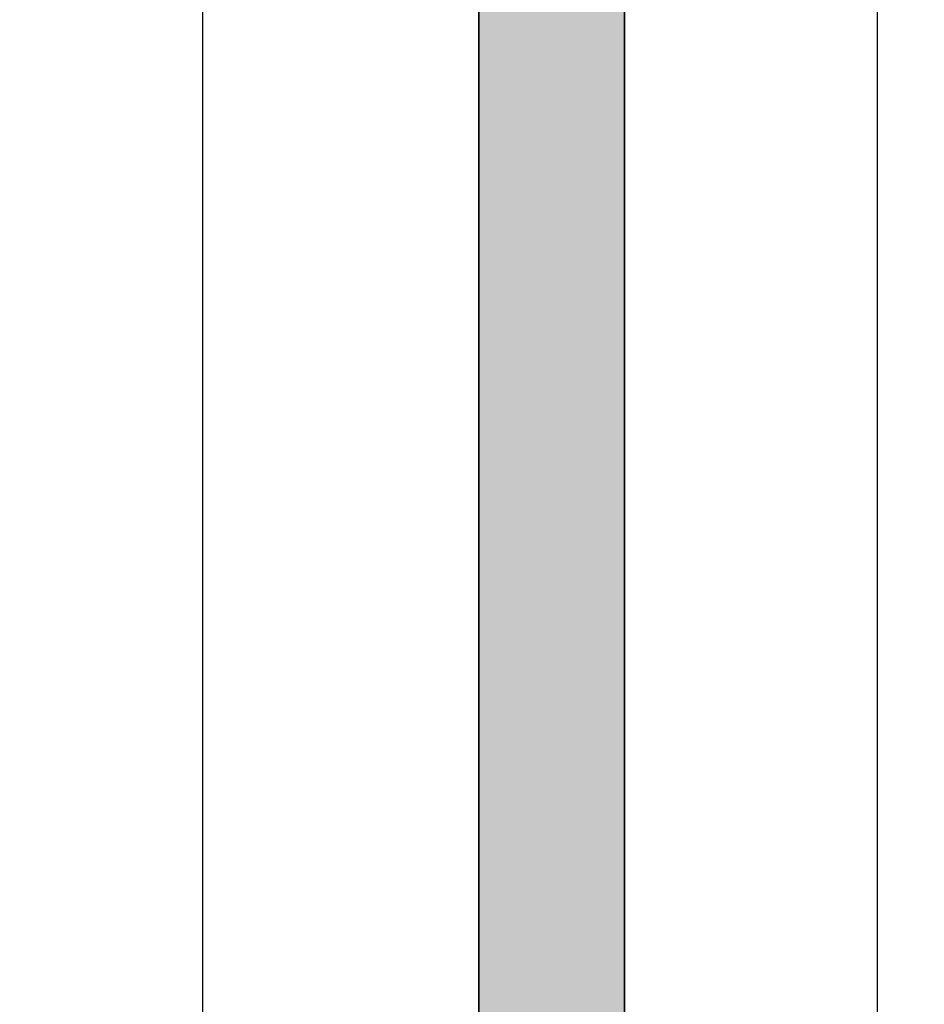
# Model space of a CAD drawing. Units: inches. Extents: x -5 to 330, y -522 to 40.
# Tile 8 of 23: x -5 to 51, y -391 to -330. Entities that reach past the tile are written whole.
import ezdxf

# ---------------------------------------------------------------- set-up
doc = ezdxf.new("R2010")
doc.units = ezdxf.units.IN
doc.header["$MEASUREMENT"] = 0
for name, color, linetype, lineweight in [('A-ANNO-DIMS', 2, 'Continuous', 18), ('A-FLOR-CASE', 8, 'Continuous', 25), ('A-WALL', 7, 'Continuous', 35)]:
    doc.layers.add(name, color=color, linetype=linetype, lineweight=lineweight)
doc.layers.add('A-WALL-PATT', color=18, linetype='Continuous', lineweight=13, true_color=0x000000)
doc.styles.get("Standard").update_dxf_attribs({"font": 'arial.ttf'})
doc.dimstyles.get("Standard").update_dxf_attribs({"dimtxt": 0.18, "dimasz": 0.18, "dimexe": 0.18, "dimexo": 0.0625, "dimgap": 0.09, "dimtad": 0, "dimtih": 1, "dimtoh": 1, "dimdec": 0, "dimzin": 0, "dimdsep": 46, "dimlunit": 3, "dimtxsty": 'Standard', "dimcen": 0.09, "dimadec": 0, "dimazin": 0, "dimtfac": 1, "dimtdec": 0, "dimtofl": 0, "dimtmove": 0, "dimatfit": 3, "dimfxl": 1, "dimtolj": 1, "dimtzin": 0, "dimarcsym": 0})

# ---------------------------------------------------------------- blocks, each defined once
blk = doc.blocks.new('*D2')
at = {"layer": 'A-ANNO-DIMS', "color": 0, "lineweight": -2, "transparency": 16777216}
for p, q in [((23.447, 12.356), (6.274, 12.356)), ((6.454, 12.176), (6.454, -203.738)), ((6.454, -425.964), (6.454, -210.049)), ((23.447, -426.144), (6.274, -426.144))]:
    blk.add_line(p, q, dxfattribs=at)
at = {"layer": 'A-ANNO-DIMS', "color": 0, "transparency": 16777216}
for points in [[(6.424, 12.176), (6.484, 12.176), (6.454, 12.356)], [(6.424, -425.964), (6.484, -425.964), (6.454, -426.144)]]:
    blk.add_solid(points, dxfattribs=at)
at = {"layer": 'Defpoints', "color": 0, "transparency": 16777216}
for p in [(23.51, 12.356), (6.454, -426.144), (23.51, -426.144)]:
    blk.add_point(p, dxfattribs=at)
at = {"layer": 'A-ANNO-DIMS', "color": 0, "transparency": 16777216, "insert": (6.454, -206.894), "char_height": 6, "attachment_point": 5}
blk.add_mtext('\\A1;36\'-7"', dxfattribs=at)
blk = doc.blocks.new('*D40')
at = {"layer": 'A-ANNO-DIMS', "color": 0, "lineweight": -2, "transparency": 16777216}
for p, q in [((32.51, -246.706), (32.51, -522.309)), ((79.01, -246.706), (79.01, -522.309)), ((32.69, -522.129), (55.151, -522.129)), ((78.83, -522.129), (56.369, -522.129))]:
    blk.add_line(p, q, dxfattribs=at)
at = {"layer": 'A-ANNO-DIMS', "color": 0, "transparency": 16777216}
for points in [[(32.69, -522.099), (32.69, -522.159), (32.51, -522.129)], [(78.83, -522.099), (78.83, -522.159), (79.01, -522.129)]]:
    blk.add_solid(points, dxfattribs=at)
at = {"layer": 'Defpoints', "color": 0, "transparency": 16777216}
for p in [(32.51, -246.644), (79.01, -246.644), (79.01, -522.129)]:
    blk.add_point(p, dxfattribs=at)
at = {"layer": 'A-ANNO-DIMS', "color": 0, "transparency": 16777216, "insert": (55.76, -522.129), "char_height": 0.18, "attachment_point": 5}
blk.add_mtext('\\A1;3\'-10 1/2"', dxfattribs=at)

msp = doc.modelspace()

# ---------------------------------------------------------------- hatches: boundary and pattern name
at = {"layer": 'A-WALL-PATT'}
h = msp.add_hatch(color=256, dxfattribs=at)
h.dxf.hatch_style = 1
h.paths.add_polyline_path([(164.01, -44.152), (159.51, -44.152), (159.51, -153.144), (164.01, -153.144)], flags=17)
h.paths.add_polyline_path([(224.01, -188.144), (272.01, -188.144), (272.01, -218.144), (260.01, -218.144), (260.01, -222.644), (272.01, -222.644), (272.01, -292.644), (159.01, -292.644), (159.01, -297.144), (272.01, -297.144), (272.01, -417.144), (245.51, -417.144), (245.51, -426.144), (272.01, -426.144), (272.01, -495.144), (281.01, -495.144), (281.01, 12.356), (23.51, 12.356), (23.51, -426.144), (62.918, -426.144), (62.918, -417.144), (32.51, -417.144), (32.51, -297.144), (48.129, -297.144), (48.129, -292.644), (32.51, -292.644), (32.51, -140.644), (133.51, -140.644), (133.51, -131.644), (32.51, -131.644), (32.51, 3.356), (159.51, 3.356), (164.01, 3.356), (220.01, 3.356), (224.51, 3.356), (272.01, 3.356), (272.01, -179.144), (159.51, -179.144), (159.51, -188.144), (219.51, -188.144), (219.51, -266.644), (224.01, -266.644), (224.01, -222.644), (236.01, -222.644), (236.01, -218.144), (224.01, -218.144)])
h.paths.add_polyline_path([(133.01, -292.644), (128.51, -292.644), (128.51, -297.144), (128.51, -417.144), (122.918, -417.144), (122.918, -426.144), (133.01, -426.144)], flags=17)
h.paths.add_polyline_path([(185.51, -417.144), (159.01, -417.144), (159.01, -426.144), (185.51, -426.144)], flags=17)
h.paths.add_polyline_path([(133.51, -140.644), (129.01, -140.644), (129.01, -246.644), (133.51, -246.644)], flags=17)
h.paths.add_polyline_path([(246.01, -48.644), (224.51, -48.644), (224.51, -27.627), (220.01, -27.627), (220.01, -48.644), (198.604, -48.644), (198.604, -53.144), (246.01, -53.144)], flags=17)

# ---------------------------------------------------------------- linework, layer by layer
at = {"layer": 'A-FLOR-CASE'}
msp.add_line((48.129, -297.144), (48.129, -393.928), dxfattribs=at)
at = {"layer": 'A-WALL'}
for p, q in [((23.51, 12.356), (23.51, -495.144)), ((32.51, -297.144), (32.51, -417.144))]:
    msp.add_line(p, q, dxfattribs=at)

# ---------------------------------------------------------------- dimensions: what is measured, and where the dimension line sits
at = {"layer": 'A-ANNO-DIMS'}
dim = msp.add_linear_dim(base=(6.454321893, -426.143582029), p1=(23.509888577, 12.356417971), p2=(23.509888577, -426.143582029), angle=90, dimstyle='Standard', override={"dimtxt": 6, "dimclrd": 0, "dimclre": 0, "dimclrt": 0}, dxfattribs=at)
dim.commit()
dim.dimension.update_dxf_attribs({"geometry": '*D2', "text_midpoint": (6.454321893, -206.893582029)})
dim = msp.add_linear_dim(base=(79.01, -522.129), p1=(32.51, -246.644), p2=(79.01, -246.644), dimstyle='Standard', override={"dimdec": 1, "dimlfac": 1, "dimrnd": 0, "dimzin": 1, "dimdsep": 46, "dimlunit": 4, "dimfrac": 2}, dxfattribs=at)
dim.commit()
dim.dimension.update_dxf_attribs({"geometry": '*D40', "text_midpoint": (55.76, -522.129)})

doc.saveas('drawing.dxf')
